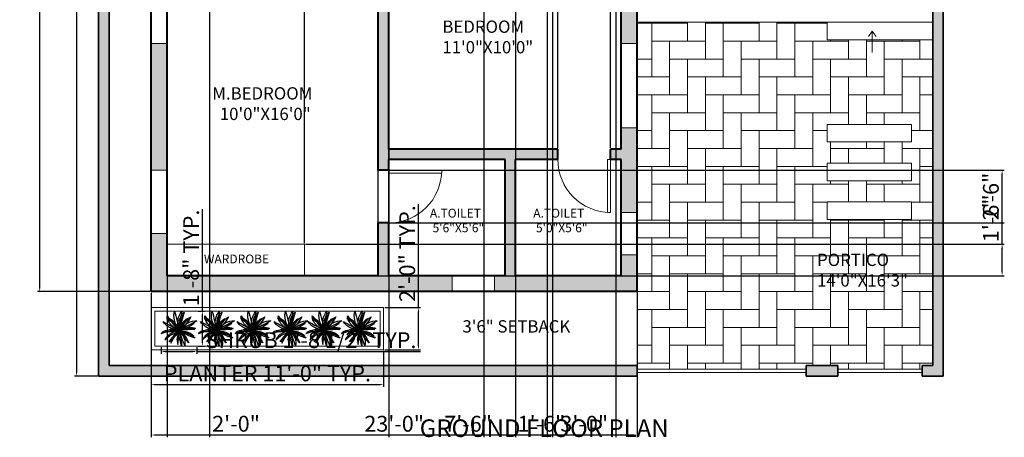
# Model space of a CAD drawing. Units: inches. Extents: x 2337 to 3570, y 1258 to 1938.
# Tile 20 of 30: x 2943 to 3502, y 1258 to 1496. Entities that reach past the tile are written whole.
import ezdxf

# ---------------------------------------------------------------- set-up
doc = ezdxf.new("R2010")
doc.units = ezdxf.units.IN
for name, color, linetype, lineweight in [('A-ANNO-DIMS', 2, 'Continuous', 18), ('A-ANNO-SYMB', 7, 'Continuous', 18), ('A-ANNO-TEXT', 7, 'Continuous', 18), ('A-ANNO-TITL', 7, 'Continuous', 30), ('A-AREA-IDEN', 7, 'Continuous', 18), ('A-DOOR', 4, 'Continuous', 20), ('A-FLOR-CASE', 34, 'Continuous', 18), ('A-FLOR-EDGE', 8, 'Continuous', 20), ('A-FLOR-PATT', 252, 'Continuous', 13), ('A-FLOR-STRS', 7, 'Continuous', 20), ('A-GLAZ', 4, 'Continuous', 18), ('A-WALL', 7, 'Continuous', 40), ('C-PROP', 7, 'Continuous', 35), ('CAY', 94, 'Continuous', 13), ('L-PLNT-BEDS', 94, 'Continuous', 20), ('L-SITE-GATE', 4, 'Continuous', 18)]:
    doc.layers.add(name, color=color, linetype=linetype, lineweight=lineweight)
doc.layers.add('A-WALL-PATT', color=18, linetype='Continuous', lineweight=13, true_color=0x000000)
doc.layers.add('C-PROP-PATT', color=251, linetype='Continuous', lineweight=13, true_color=0x636466)
doc.layers.add('DIENHOA', color=3, linetype='Continuous')
doc.styles.get("Standard").update_dxf_attribs({"font": 'arial.ttf'})
doc.dimstyles.new('ISO-25', dxfattribs={"dimtxt": 9, "dimasz": 2.5, "dimexe": 1.25, "dimexo": 0.625, "dimtad": 1, "dimdec": 1, "dimlunit": 3, "dimtxsty": 'Standard', "dimcen": 2.5, "dimadec": 0, "dimazin": 0, "dimtfac": 1, "dimtdec": 1, "dimtmove": 0, "dimatfit": 3, "dimfxl": 1, "dimarcsym": 0})

# ---------------------------------------------------------------- blocks, each defined once
blk = doc.blocks.new('*U3')
for p, q in [((0, 0), (0, -6)), ((30, 0), (30, -6))]:
    blk.add_line(p, q)
blk.add_lwpolyline([(0, 0), (0, 30), (1.75, 30), (1.75, 0)], close=True)
blk.add_arc((0, 0), 30, 0, 90)
blk = doc.blocks.new('*D5')
at = {"layer": 'A-ANNO-DIMS', "color": 0, "lineweight": -2, "transparency": 16777216}
for p, q in [((2987.16, 1893.12), (2974.1, 1893.12)), ((2975.35, 1890.62), (2975.35, 1295.62)), ((2987.16, 1293.12), (2974.1, 1293.12))]:
    blk.add_line(p, q, dxfattribs=at)
at = {"layer": 'A-ANNO-DIMS', "color": 0, "transparency": 16777216}
for points in [[(2974.93, 1890.62), (2975.77, 1890.62), (2975.35, 1893.12)], [(2974.93, 1295.62), (2975.77, 1295.62), (2975.35, 1293.12)]]:
    blk.add_solid(points, dxfattribs=at)
at = {"layer": 'Defpoints', "color": 0, "transparency": 16777216}
for p in [(2987.79, 1893.12), (2975.35, 1293.12), (2987.79, 1293.12)]:
    blk.add_point(p, dxfattribs=at)
at = {"layer": 'A-ANNO-DIMS', "color": 0, "transparency": 16777216, "insert": (2970.13, 1593.12), "char_height": 9, "attachment_point": 5, "rotation": 90}
blk.add_mtext("50'", dxfattribs=at)
blk = doc.blocks.new('Cay03_mb')
at = {"layer": 'DIENHOA'}
for p, q in [((-365, 390), (-414, 403)), ((-414, 403), (-240, 278)), ((-315, 371), (-365, 390)), ((-264, 343), (-315, 371)), ((-211, 305), (-264, 343)), ((10, 295), (25, 374)), ((25, 374), (49, 444)), ((49, 444), (79, 504)), ((97, 366), (76, 291)), ((79, 504), (119, 555)), ((119, 442), (97, 366)), ((119, 555), (166, 599)), ((142, 519), (119, 442)), ((166, 599), (142, 519)), ((-345, 5), (-400, -17)), ((-299, 20), (-345, 5)), ((-255, 27), (-299, 20)), ((-208, 28), (-255, 27)), ((-240, 278), (-88, 95)), ((-158, 252), (-211, 305)), ((-153, 22), (-208, 28)), ((-104, 184), (-158, 252)), ((-83, 10), (-153, 22)), ((-50, 98), (-104, 184)), ((-88, 95), (5, -8)), ((5, -8), (-83, 10)), ((5, -8), (-50, 98)), ((0, 105), (2, 206)), ((5, -8), (0, 105)), ((2, 206), (10, 295)), ((5, -8), (76, 75)), ((20, 68), (5, -8)), ((75, 36), (5, -8)), ((5, -8), (100, 18)), ((46, 1), (5, -8)), ((37, 142), (20, 68)), ((56, 216), (37, 142)), ((97, 7), (46, 1)), ((76, 291), (56, 216)), ((145, 77), (75, 36)), ((76, 75), (147, 144)), ((155, 12), (97, 7)), ((100, 18), (182, 37)), ((217, 117), (145, 77)), ((147, 144), (219, 200)), ((220, 15), (155, 12)), ((182, 37), (253, 49)), ((290, 155), (217, 117)), ((219, 200), (291, 243)), ((289, 17), (220, 15)), ((253, 49), (315, 54)), ((362, 19), (289, 17)), ((364, 193), (290, 155)), ((291, 243), (363, 275)), ((315, 54), (369, 53)), ((436, 19), (362, 19)), ((363, 275), (437, 297)), ((438, 231), (364, 193)), ((369, 53), (419, 47)), ((419, 47), (465, 35)), ((510, 19), (436, 19)), ((437, 297), (511, 310)), ((512, 271), (438, 231)), ((465, 35), (510, 19)), ((511, 310), (586, 314)), ((586, 314), (512, 271)), ((-400, -17), (-468, -48)), ((-468, -48), (-376, -38)), ((-376, -38), (-295, -28)), ((-330, -387), (-271, -307)), ((-295, -28), (-226, -19)), ((-250, -318), (-291, -355)), ((-271, -307), (-216, -236)), ((-206, -276), (-250, -318)), ((-226, -19), (-166, -11)), ((-216, -236), (-166, -174)), ((-162, -231), (-206, -276)), ((-166, -11), (-114, -6)), ((-166, -174), (-120, -122)), ((-118, -181), (-162, -231)), ((-120, -122), (-80, -80)), ((-75, -127), (-118, -181)), ((-114, -6), (-69, -3)), ((-80, -80), (-45, -46)), ((-33, -69), (-75, -127)), ((-69, -3), (-30, -3)), ((-45, -46), (-17, -22)), ((5, -8), (-33, -69)), ((-30, -3), (5, -8)), ((-17, -22), (5, -8)), ((5, -8), (57, -73)), ((26, -64), (5, -8)), ((5, -8), (113, -40)), ((53, -42), (5, -8)), ((47, -126), (26, -64)), ((69, -191), (47, -126)), ((107, -76), (53, -42)), ((57, -73), (100, -139)), ((91, -257), (69, -191)), ((113, -322), (91, -257)), ((100, -139), (136, -204)), ((166, -110), (107, -76)), ((113, -40), (207, -74)), ((135, -386), (113, -322)), ((136, -204), (163, -268)), ((163, -268), (181, -330)), ((229, -143), (166, -110)), ((207, -74), (290, -108)), ((296, -175), (229, -143)), ((290, -108), (359, -141)), ((367, -205), (296, -175)), ((359, -141), (417, -174)), ((442, -233), (367, -205)), ((417, -174), (463, -204)), ((519, -258), (442, -233)), ((463, -204), (496, -232)), ((496, -232), (519, -258)), ((-291, -355), (-330, -387)), ((158, -445), (135, -386)), ((180, -499), (158, -445)), ((190, -446), (180, -499)), ((181, -330), (190, -390)), ((190, -390), (190, -446))]:
    blk.add_line(p, q, dxfattribs=at)
for points in [[(-396, 474), (-348, 406), (-301, 339), (-254, 275), (-208, 212), (-162, 151), (-115, 91), (-66, 32), (-16, -27)], [(-16, -27), (-108, 39), (-187, 102), (-252, 163), (-305, 224), (-345, 285), (-374, 347), (-390, 409), (-396, 474)], [(24, -5), (-41, 82), (-92, 167), (-130, 249), (-156, 330), (-170, 408), (-175, 484), (-170, 559), (-157, 633)], [(-157, 633), (-132, 551), (-111, 470), (-90, 389), (-70, 309), (-49, 229), (-27, 150), (-3, 72), (24, -5)], [(-16, -27), (-38, 80), (-49, 178), (-49, 269), (-39, 353), (-19, 430), (9, 501), (45, 567), (88, 629)], [(88, 629), (75, 544), (61, 461), (46, 379), (31, 298), (16, 217), (3, 136), (-8, 55), (-16, -27)], [(273, 387), (228, 329), (182, 270), (138, 212), (97, 156), (60, 103), (28, 55), (2, 11), (-16, -27)], [(-16, -27), (21, 64), (57, 140), (91, 203), (125, 255), (160, 297), (195, 332), (233, 362), (273, 387)], [(24, -5), (20, 93), (20, 177), (25, 249), (34, 310), (47, 363), (65, 409), (87, 452), (113, 492)], [(113, 492), (96, 420), (79, 347), (64, 276), (50, 208), (38, 145), (30, 87), (25, 36), (24, -5)], [(384, 437), (342, 368), (298, 302), (253, 239), (206, 181), (159, 127), (113, 78), (68, 34), (24, -5)], [(24, -5), (80, 92), (134, 176), (186, 248), (234, 309), (279, 357), (319, 395), (355, 421), (384, 437)], [(-16, -27), (-134, -5), (-235, 5), (-322, 5), (-396, -5), (-459, -22), (-512, -46), (-558, -74), (-598, -105)], [(-530, 290), (-458, 248), (-388, 208), (-319, 169), (-251, 131), (-183, 95), (-115, 60), (-46, 26), (24, -5)], [(24, -5), (-87, 15), (-185, 40), (-270, 68), (-344, 101), (-406, 140), (-457, 184), (-499, 233), (-530, 290)], [(497, 224), (429, 178), (362, 137), (294, 99), (227, 66), (162, 37), (100, 11), (40, -10), (-16, -27)], [(-16, -27), (75, 38), (160, 92), (237, 136), (307, 170), (368, 195), (420, 213), (463, 222), (497, 224)], [(24, -5), (99, 30), (173, 57), (245, 77), (313, 88), (378, 92), (438, 87), (493, 74), (541, 52)], [(541, 52), (484, 43), (421, 35), (354, 28), (285, 21), (216, 14), (148, 8), (83, 2), (24, -5)], [(-598, -105), (-393, -44), (-155, -37), (-16, -27)], [(-472, -320), (-310, -179), (-98, -73), (24, -5)], [(24, -5), (-92, -35), (-188, -68), (-267, -105), (-330, -145), (-380, -187), (-418, -231), (-448, -275), (-472, -320)], [(-276, -424), (-227, -345), (-186, -276), (-150, -216), (-119, -164), (-91, -120), (-66, -82), (-41, -52), (-16, -27)], [(-16, -27), (-85, -86), (-137, -133), (-176, -173), (-204, -210), (-226, -249), (-243, -295), (-258, -352), (-276, -424)], [(24, -5), (-14, -88), (-41, -153), (-60, -205), (-70, -251), (-73, -295), (-69, -344), (-60, -402), (-45, -475)], [(-45, -475), (-34, -383), (-25, -303), (-18, -233), (-12, -173), (-6, -121), (2, -77), (11, -39), (24, -5)], [(76, -524), (49, -428), (27, -342), (9, -264), (-4, -196), (-12, -138), (-17, -90), (-18, -53), (-16, -27)], [(478, -192), (422, -176), (361, -157), (298, -135), (232, -113), (167, -89), (102, -67), (41, -45), (-16, -27)], [(-16, -27), (67, -27), (146, -33), (219, -45), (286, -63), (346, -87), (398, -117), (443, -152), (478, -192)], [(-16, -27), (8, -95), (29, -163), (44, -231), (56, -296), (65, -359), (71, -419), (74, -474), (76, -524)], [(316, -418), (251, -343), (195, -273), (147, -210), (106, -154), (74, -105), (50, -63), (33, -30), (24, -5)], [(24, -5), (75, -57), (122, -111), (164, -165), (203, -219), (237, -273), (267, -324), (294, -373), (316, -418)]]:
    blk.add_lwpolyline(points, dxfattribs=at)
blk = doc.blocks.new('STAIR-UP-ARROW')
for p, q in [((2.25, 12), (2.25, 0)), ((2.25, 0), (0, 3.01)), ((2.25, 0), (4.5, 3.01))]:
    blk.add_line(p, q)
blk = doc.blocks.new('PLANTER-132X24IN')
for points in [[(0, 24), (132, 24), (132, 0), (0, 0)], [(2, 22), (130, 22), (130, 2), (2, 2)]]:
    blk.add_lwpolyline(points, close=True)
blk = doc.blocks.new('*D46')
at = {"layer": 'A-ANNO-DIMS', "color": 0, "lineweight": -2, "transparency": 16777216}
for p, q in [((3023.35, 1309.55), (3023.35, 1305.87)), ((3043.75, 1309.55), (3043.75, 1305.87)), ((3025.85, 1307.12), (3041.25, 1307.12)), ((3043.75, 1307.12), (3170.8, 1307.12))]:
    blk.add_line(p, q, dxfattribs=at)
at = {"layer": 'A-ANNO-DIMS', "color": 0, "transparency": 16777216}
for points in [[(3025.85, 1307.54), (3025.85, 1306.7), (3023.35, 1307.12)], [(3041.25, 1307.54), (3041.25, 1306.7), (3043.75, 1307.12)]]:
    blk.add_solid(points, dxfattribs=at)
at = {"layer": 'Defpoints', "color": 0, "transparency": 16777216}
for p in [(3023.35, 1310.18), (3043.75, 1310.18), (3043.75, 1307.12)]:
    blk.add_point(p, dxfattribs=at)
at = {"layer": 'A-ANNO-DIMS', "color": 0, "transparency": 16777216, "insert": (3108.53, 1312.4), "char_height": 9, "attachment_point": 5}
blk.add_mtext('SHRUB 1\'-8 1/2" TYP.', dxfattribs=at)
blk = doc.blocks.new('*D47')
at = {"layer": 'A-ANNO-DIMS', "color": 0, "lineweight": -2, "transparency": 16777216}
for p, q in [((3046.81, 1330.12), (3046.81, 1387.88)), ((3044.38, 1330.12), (3048.06, 1330.12)), ((3046.81, 1312.68), (3046.81, 1327.62)), ((3044.38, 1310.18), (3048.06, 1310.18))]:
    blk.add_line(p, q, dxfattribs=at)
at = {"layer": 'A-ANNO-DIMS', "color": 0, "transparency": 16777216}
for points in [[(3046.4, 1327.62), (3047.23, 1327.62), (3046.81, 1330.12)], [(3046.4, 1312.68), (3047.23, 1312.68), (3046.81, 1310.18)]]:
    blk.add_solid(points, dxfattribs=at)
at = {"layer": 'Defpoints', "color": 0, "transparency": 16777216}
for p in [(3043.75, 1330.12), (3046.81, 1330.12), (3043.75, 1310.18)]:
    blk.add_point(p, dxfattribs=at)
at = {"layer": 'A-ANNO-DIMS', "color": 0, "transparency": 16777216, "insert": (3041.59, 1360.25), "char_height": 9, "attachment_point": 5, "rotation": 90}
blk.add_mtext('1\'-8" TYP.', dxfattribs=at)
blk = doc.blocks.new('*D74')
at = {"layer": 'A-ANNO-DIMS', "color": 0, "lineweight": -2, "transparency": 16777216}
for p, q in [((3017.79, 1307.49), (3017.79, 1287.07)), ((3149.79, 1307.49), (3149.79, 1287.07)), ((3020.29, 1288.32), (3147.29, 1288.32))]:
    blk.add_line(p, q, dxfattribs=at)
at = {"layer": 'A-ANNO-DIMS', "color": 0, "transparency": 16777216}
for points in [[(3020.29, 1288.73), (3020.29, 1287.9), (3017.79, 1288.32)], [(3147.29, 1288.73), (3147.29, 1287.9), (3149.79, 1288.32)]]:
    blk.add_solid(points, dxfattribs=at)
at = {"layer": 'Defpoints', "color": 0, "transparency": 16777216}
for p in [(3017.79, 1308.12), (3149.79, 1308.12), (3149.79, 1288.32)]:
    blk.add_point(p, dxfattribs=at)
at = {"layer": 'A-ANNO-DIMS', "color": 0, "transparency": 16777216, "insert": (3083.79, 1293.54), "char_height": 9, "attachment_point": 5}
blk.add_mtext('PLANTER 11\'-0" TYP.', dxfattribs=at)
blk = doc.blocks.new('*D75')
at = {"layer": 'A-ANNO-DIMS', "color": 0, "lineweight": -2, "transparency": 16777216}
for p, q in [((3169.59, 1332.12), (3169.59, 1390.88)), ((3150.41, 1332.12), (3170.84, 1332.12)), ((3169.59, 1310.62), (3169.59, 1329.62)), ((3150.41, 1308.12), (3170.84, 1308.12))]:
    blk.add_line(p, q, dxfattribs=at)
at = {"layer": 'A-ANNO-DIMS', "color": 0, "transparency": 16777216}
for points in [[(3169.17, 1329.62), (3170, 1329.62), (3169.59, 1332.12)], [(3169.17, 1310.62), (3170, 1310.62), (3169.59, 1308.12)]]:
    blk.add_solid(points, dxfattribs=at)
at = {"layer": 'Defpoints', "color": 0, "transparency": 16777216}
for p in [(3149.79, 1332.12), (3169.59, 1332.12), (3149.79, 1308.12)]:
    blk.add_point(p, dxfattribs=at)
at = {"layer": 'A-ANNO-DIMS', "color": 0, "transparency": 16777216, "insert": (3164.37, 1362.75), "char_height": 9, "attachment_point": 5, "rotation": 90}
blk.add_mtext('2\'-0" TYP.', dxfattribs=at)
blk = doc.blocks.new('*D100')
at = {"layer": 'A-ANNO-DIMS', "color": 0, "lineweight": -2, "transparency": 16777216}
for p, q in [((3248.79, 1422.74), (3248.79, 1927.77)), ((3251.29, 1926.52), (3276.29, 1926.52)), ((3278.79, 1422.74), (3278.79, 1927.77))]:
    blk.add_line(p, q, dxfattribs=at)
at = {"layer": 'A-ANNO-DIMS', "color": 0, "transparency": 16777216}
for points in [[(3251.29, 1926.93), (3251.29, 1926.1), (3248.79, 1926.52)], [(3276.29, 1926.93), (3276.29, 1926.1), (3278.79, 1926.52)]]:
    blk.add_solid(points, dxfattribs=at)
at = {"layer": 'Defpoints', "color": 0, "transparency": 16777216}
for p in [(3278.79, 1926.52), (3248.79, 1422.12), (3278.79, 1422.12)]:
    blk.add_point(p, dxfattribs=at)
at = {"layer": 'A-ANNO-DIMS', "color": 0, "transparency": 16777216, "insert": (3263.79, 1931.74), "char_height": 9, "attachment_point": 5}
blk.add_mtext('2\'-6"', dxfattribs=at)
blk = doc.blocks.new('*D101')
at = {"layer": 'A-ANNO-DIMS', "color": 0, "lineweight": -2, "transparency": 16777216}
for p, q in [((3147.41, 1410.12), (3502.44, 1410.12)), ((3501.19, 1382.62), (3501.19, 1407.62)), ((3147.41, 1380.12), (3502.44, 1380.12))]:
    blk.add_line(p, q, dxfattribs=at)
at = {"layer": 'A-ANNO-DIMS', "color": 0, "transparency": 16777216}
for points in [[(3500.77, 1407.62), (3501.6, 1407.62), (3501.19, 1410.12)], [(3500.77, 1382.62), (3501.6, 1382.62), (3501.19, 1380.12)]]:
    blk.add_solid(points, dxfattribs=at)
at = {"layer": 'Defpoints', "color": 0, "transparency": 16777216}
for p in [(3146.79, 1410.12), (3501.19, 1410.12), (3146.79, 1380.12)]:
    blk.add_point(p, dxfattribs=at)
at = {"layer": 'A-ANNO-DIMS', "color": 0, "transparency": 16777216, "insert": (3495.97, 1395.12), "char_height": 9, "attachment_point": 5, "rotation": 90}
blk.add_mtext('2\'-6"', dxfattribs=at)
blk = doc.blocks.new('*D102')
at = {"layer": 'A-ANNO-DIMS', "color": 0, "lineweight": -2, "transparency": 16777216}
for p, q in [((3245.79, 1763.49), (3245.79, 1258.47)), ((3281.79, 1763.49), (3281.79, 1258.47)), ((3248.29, 1259.72), (3279.29, 1259.72))]:
    blk.add_line(p, q, dxfattribs=at)
at = {"layer": 'A-ANNO-DIMS', "color": 0, "transparency": 16777216}
for points in [[(3248.29, 1260.13), (3248.29, 1259.3), (3245.79, 1259.72)], [(3279.29, 1260.13), (3279.29, 1259.3), (3281.79, 1259.72)]]:
    blk.add_solid(points, dxfattribs=at)
at = {"layer": 'Defpoints', "color": 0, "transparency": 16777216}
for p in [(3245.79, 1764.12), (3281.79, 1764.12), (3281.79, 1259.72)]:
    blk.add_point(p, dxfattribs=at)
at = {"layer": 'A-ANNO-DIMS', "color": 0, "transparency": 16777216, "insert": (3263.79, 1264.94), "char_height": 9, "attachment_point": 5}
blk.add_mtext('3\'-0"', dxfattribs=at)
blk = doc.blocks.new('*D104')
at = {"layer": 'A-ANNO-DIMS', "color": 0, "lineweight": -2, "transparency": 16777216}
for p, q in [((3144.29, 1926.52), (3141.79, 1926.52)), ((3146.79, 1350.74), (3146.79, 1927.77)), ((3146.79, 1926.52), (3152.79, 1926.52)), ((3152.79, 1350.74), (3152.79, 1927.77)), ((3155.29, 1926.52), (3182.96, 1926.52))]:
    blk.add_line(p, q, dxfattribs=at)
at = {"layer": 'A-ANNO-DIMS', "color": 0, "transparency": 16777216}
for points in [[(3144.29, 1926.93), (3144.29, 1926.1), (3146.79, 1926.52)], [(3155.29, 1926.93), (3155.29, 1926.1), (3152.79, 1926.52)]]:
    blk.add_solid(points, dxfattribs=at)
at = {"layer": 'Defpoints', "color": 0, "transparency": 16777216}
for p in [(3152.79, 1926.52), (3146.79, 1350.12), (3152.79, 1350.12)]:
    blk.add_point(p, dxfattribs=at)
at = {"layer": 'A-ANNO-DIMS', "color": 0, "transparency": 16777216, "insert": (3170.37, 1931.74), "char_height": 9, "attachment_point": 5}
blk.add_mtext('0\'-6"', dxfattribs=at)
blk = doc.blocks.new('*D105')
at = {"layer": 'A-ANNO-DIMS', "color": 0, "lineweight": -2, "transparency": 16777216}
for p, q in [((3026.79, 1640.49), (3026.79, 1258.47)), ((3050.79, 1640.49), (3050.79, 1258.47)), ((3029.29, 1259.72), (3048.29, 1259.72)), ((3050.79, 1259.72), (3078.61, 1259.72))]:
    blk.add_line(p, q, dxfattribs=at)
at = {"layer": 'A-ANNO-DIMS', "color": 0, "transparency": 16777216}
for points in [[(3029.29, 1260.13), (3029.29, 1259.3), (3026.79, 1259.72)], [(3048.29, 1260.13), (3048.29, 1259.3), (3050.79, 1259.72)]]:
    blk.add_solid(points, dxfattribs=at)
at = {"layer": 'Defpoints', "color": 0, "transparency": 16777216}
for p in [(3026.79, 1641.12), (3050.79, 1641.12), (3050.79, 1259.72)]:
    blk.add_point(p, dxfattribs=at)
at = {"layer": 'A-ANNO-DIMS', "color": 0, "transparency": 16777216, "insert": (3065.95, 1264.94), "char_height": 9, "attachment_point": 5}
blk.add_mtext('2\'-0"', dxfattribs=at)
blk = doc.blocks.new('*D109')
at = {"layer": 'A-ANNO-DIMS', "color": 0, "lineweight": -2, "transparency": 16777216}
for p, q in [((3017.79, 1340.49), (3017.79, 1258.47)), ((3293.79, 1340.49), (3293.79, 1258.47)), ((3020.29, 1259.72), (3291.29, 1259.72))]:
    blk.add_line(p, q, dxfattribs=at)
at = {"layer": 'A-ANNO-DIMS', "color": 0, "transparency": 16777216}
for points in [[(3020.29, 1260.13), (3020.29, 1259.3), (3017.79, 1259.72)], [(3291.29, 1260.13), (3291.29, 1259.3), (3293.79, 1259.72)]]:
    blk.add_solid(points, dxfattribs=at)
at = {"layer": 'Defpoints', "color": 0, "transparency": 16777216}
for p in [(3017.79, 1341.12), (3293.79, 1341.12), (3293.79, 1259.72)]:
    blk.add_point(p, dxfattribs=at)
at = {"layer": 'A-ANNO-DIMS', "color": 0, "transparency": 16777216, "insert": (3155.79, 1264.94), "char_height": 9, "attachment_point": 5}
blk.add_mtext('23\'-0"', dxfattribs=at)
blk = doc.blocks.new('*D110')
at = {"layer": 'A-ANNO-DIMS', "color": 0, "lineweight": -2, "transparency": 16777216}
for p, q in [((3017.16, 1857.12), (2953.14, 1857.12)), ((2954.39, 1343.62), (2954.39, 1854.62)), ((3017.16, 1341.12), (2953.14, 1341.12))]:
    blk.add_line(p, q, dxfattribs=at)
at = {"layer": 'A-ANNO-DIMS', "color": 0, "transparency": 16777216}
for points in [[(2953.97, 1854.62), (2954.8, 1854.62), (2954.39, 1857.12)], [(2953.97, 1343.62), (2954.8, 1343.62), (2954.39, 1341.12)]]:
    blk.add_solid(points, dxfattribs=at)
at = {"layer": 'Defpoints', "color": 0, "transparency": 16777216}
for p in [(2954.39, 1857.12), (3017.79, 1857.12), (3017.79, 1341.12)]:
    blk.add_point(p, dxfattribs=at)
at = {"layer": 'A-ANNO-DIMS', "color": 0, "transparency": 16777216, "insert": (2949.16, 1599.12), "char_height": 9, "attachment_point": 5, "rotation": 90}
blk.add_mtext('43\'-0"', dxfattribs=at)
blk = doc.blocks.new('*D112')
at = {"layer": 'A-ANNO-DIMS', "color": 0, "lineweight": -2, "transparency": 16777216}
for p, q in [((3026.79, 1368.74), (3026.79, 1927.77)), ((3029.29, 1926.52), (3102.29, 1926.52)), ((3104.79, 1368.74), (3104.79, 1927.77))]:
    blk.add_line(p, q, dxfattribs=at)
at = {"layer": 'A-ANNO-DIMS', "color": 0, "transparency": 16777216}
for points in [[(3029.29, 1926.93), (3029.29, 1926.1), (3026.79, 1926.52)], [(3102.29, 1926.93), (3102.29, 1926.1), (3104.79, 1926.52)]]:
    blk.add_solid(points, dxfattribs=at)
at = {"layer": 'Defpoints', "color": 0, "transparency": 16777216}
for p in [(3104.79, 1926.52), (3026.79, 1368.12), (3104.79, 1368.12)]:
    blk.add_point(p, dxfattribs=at)
at = {"layer": 'A-ANNO-DIMS', "color": 0, "transparency": 16777216, "insert": (3065.79, 1931.74), "char_height": 9, "attachment_point": 5}
blk.add_mtext('6\'-6"', dxfattribs=at)
blk = doc.blocks.new('*D113')
at = {"layer": 'A-ANNO-DIMS', "color": 0, "lineweight": -2, "transparency": 16777216}
for p, q in [((3501.19, 1368.12), (3501.19, 1394.94)), ((3105.41, 1368.12), (3502.44, 1368.12)), ((3501.19, 1352.62), (3501.19, 1365.62)), ((3105.41, 1350.12), (3502.44, 1350.12))]:
    blk.add_line(p, q, dxfattribs=at)
at = {"layer": 'A-ANNO-DIMS', "color": 0, "transparency": 16777216}
for points in [[(3500.77, 1365.62), (3501.6, 1365.62), (3501.19, 1368.12)], [(3500.77, 1352.62), (3501.6, 1352.62), (3501.19, 1350.12)]]:
    blk.add_solid(points, dxfattribs=at)
at = {"layer": 'Defpoints', "color": 0, "transparency": 16777216}
for p in [(3104.79, 1368.12), (3501.19, 1368.12), (3104.79, 1350.12)]:
    blk.add_point(p, dxfattribs=at)
at = {"layer": 'A-ANNO-DIMS', "color": 0, "transparency": 16777216, "insert": (3495.97, 1382.78), "char_height": 9, "attachment_point": 5, "rotation": 90}
blk.add_mtext('1\'-6"', dxfattribs=at)
blk = doc.blocks.new('*D114')
at = {"layer": 'A-ANNO-DIMS', "color": 0, "lineweight": -2, "transparency": 16777216}
for p, q in [((3152.79, 1523.49), (3152.79, 1258.47)), ((3242.79, 1523.49), (3242.79, 1258.47)), ((3155.29, 1259.72), (3240.29, 1259.72))]:
    blk.add_line(p, q, dxfattribs=at)
at = {"layer": 'A-ANNO-DIMS', "color": 0, "transparency": 16777216}
for points in [[(3155.29, 1260.13), (3155.29, 1259.3), (3152.79, 1259.72)], [(3240.29, 1260.13), (3240.29, 1259.3), (3242.79, 1259.72)]]:
    blk.add_solid(points, dxfattribs=at)
at = {"layer": 'Defpoints', "color": 0, "transparency": 16777216}
for p in [(3152.79, 1524.12), (3242.79, 1524.12), (3242.79, 1259.72)]:
    blk.add_point(p, dxfattribs=at)
at = {"layer": 'A-ANNO-DIMS', "color": 0, "transparency": 16777216, "insert": (3197.79, 1264.94), "char_height": 9, "attachment_point": 5}
blk.add_mtext('7\'-6"', dxfattribs=at)
blk = doc.blocks.new('*D117')
at = {"layer": 'A-ANNO-DIMS', "color": 0, "lineweight": -2, "transparency": 16777216}
for p, q in [((3206.79, 1604.49), (3206.79, 1258.47)), ((3224.79, 1604.49), (3224.79, 1258.47)), ((3209.29, 1259.72), (3222.29, 1259.72)), ((3224.79, 1259.72), (3251.61, 1259.72))]:
    blk.add_line(p, q, dxfattribs=at)
at = {"layer": 'A-ANNO-DIMS', "color": 0, "transparency": 16777216}
for points in [[(3209.29, 1260.13), (3209.29, 1259.3), (3206.79, 1259.72)], [(3222.29, 1260.13), (3222.29, 1259.3), (3224.79, 1259.72)]]:
    blk.add_solid(points, dxfattribs=at)
at = {"layer": 'Defpoints', "color": 0, "transparency": 16777216}
for p in [(3206.79, 1605.12), (3224.79, 1605.12), (3224.79, 1259.72)]:
    blk.add_point(p, dxfattribs=at)
at = {"layer": 'A-ANNO-DIMS', "color": 0, "transparency": 16777216, "insert": (3239.45, 1264.94), "char_height": 9, "attachment_point": 5}
blk.add_mtext('1\'-6"', dxfattribs=at)

msp = doc.modelspace()

# ---------------------------------------------------------------- hatches: boundary and pattern name
at = {"layer": 'A-FLOR-PATT'}
h = msp.add_hatch(dxfattribs=at)
h.set_pattern_fill('AR-HBONE', color=256, scale=0.1, angle=45)
h.set_pattern_definition([(90, (-558.681, 0), (-10.16, 10.16), [30.48, -10.16]), (180, (-558.681, 10.16), (-10.16, 10.16), [30.48, -10.16])])
h.paths.add_polyline_path([(3461.79, 1484.12), (3401.79, 1484.12), (3401.79, 1494.12), (3293.79, 1494.12), (3293.79, 1341.12), (3293.79, 1299.12), (3293.79, 1297.12), (3389.79, 1297.12), (3389.79, 1299.12), (3407.79, 1299.12), (3407.79, 1297.12), (3455.79, 1297.12), (3455.79, 1299.12), (3461.79, 1299.12)])
h.paths.add_polyline_path([(3401.79, 1426.12), (3401.79, 1436.12), (3449.79, 1436.12), (3449.79, 1426.12)], flags=16)
h.paths.add_polyline_path([(3401.79, 1414.12), (3449.79, 1414.12), (3449.79, 1404.12), (3401.79, 1404.12)], flags=16)
h.paths.add_polyline_path([(3401.79, 1392.12), (3449.79, 1392.12), (3449.79, 1382.12), (3401.79, 1382.12)], flags=16)
h.paths.add_polyline_path([(3393.24, 1340.04), (3446.57, 1340.04), (3446.57, 1366.16), (3393.24, 1366.16)], flags=24)
at = {"layer": 'A-WALL-PATT'}
h = msp.add_hatch(color=256, dxfattribs=at)
h.dxf.hatch_style = 1
h.paths.add_polyline_path([(3233.79, 1857.12), (3017.79, 1857.12), (3017.79, 1824.12), (3026.79, 1824.12), (3026.79, 1848.12), (3233.79, 1848.12)])
h.paths.add_polyline_path([(3128.79, 1764.12), (3026.79, 1764.12), (3026.79, 1788.12), (3017.79, 1788.12), (3017.79, 1743.12), (3026.79, 1743.12), (3026.79, 1755.12), (3128.79, 1755.12)])
h.paths.add_polyline_path([(3245.79, 1761.12), (3245.79, 1764.12), (3164.79, 1764.12), (3164.79, 1755.12), (3170.79, 1755.12), (3170.79, 1701.12), (3224.79, 1701.12), (3224.79, 1605.12), (3233.79, 1605.12), (3233.79, 1713.12), (3224.79, 1713.12), (3224.79, 1707.12), (3176.79, 1707.12), (3176.79, 1755.12), (3224.79, 1755.12), (3224.79, 1749.12), (3233.79, 1749.12), (3233.79, 1755.12), (3245.79, 1755.12)])
h.paths.add_polyline_path([(3026.79, 1707.12), (3017.79, 1707.12), (3017.79, 1617.12), (3026.79, 1617.12), (3026.79, 1635.12), (3068.79, 1635.12), (3068.79, 1641.12), (3026.79, 1641.12)])
h.paths.add_polyline_path([(3104.79, 1551.12), (3026.79, 1551.12), (3026.79, 1569.12), (3017.79, 1569.12), (3017.79, 1518.12), (3026.79, 1518.12), (3026.79, 1542.12), (3104.79, 1542.12)])
h.paths.add_polyline_path([(3026.79, 1482.12), (3017.79, 1482.12), (3017.79, 1410.12), (3026.79, 1410.12)])
h.paths.add_polyline_path([(3188.79, 1350.12), (3152.79, 1350.12), (3152.79, 1380.12), (3146.79, 1380.12), (3146.79, 1350.12), (3026.79, 1350.12), (3026.79, 1374.12), (3017.79, 1374.12), (3017.79, 1341.12), (3188.79, 1341.12)])
h.paths.add_polyline_path([(3224.79, 1416.12), (3248.79, 1416.12), (3248.79, 1422.12), (3152.79, 1422.12), (3152.79, 1542.12), (3242.79, 1542.12), (3242.79, 1551.12), (3233.79, 1551.12), (3233.79, 1557.12), (3224.79, 1557.12), (3224.79, 1551.12), (3140.79, 1551.12), (3140.79, 1542.12), (3146.79, 1542.12), (3146.79, 1410.12), (3152.79, 1410.12), (3152.79, 1416.12), (3218.79, 1416.12), (3218.79, 1350.12), (3212.79, 1350.12), (3212.79, 1341.12), (3293.79, 1341.12), (3293.79, 1362.12), (3284.79, 1362.12), (3284.79, 1350.12), (3224.79, 1350.12)])
h.paths.add_polyline_path([(3293.79, 1434.12), (3284.79, 1434.12), (3284.79, 1422.12), (3278.79, 1422.12), (3278.79, 1416.12), (3284.79, 1416.12), (3284.79, 1386.12), (3293.79, 1386.12)], flags=17)
h.paths.add_polyline_path([(3293.79, 1542.12), (3314.79, 1542.12), (3314.79, 1551.12), (3278.79, 1551.12), (3278.79, 1545.12), (3278.79, 1542.12), (3284.79, 1542.12), (3284.79, 1482.12), (3293.79, 1482.12)])
h.paths.add_polyline_path([(3371.79, 1551.12), (3350.79, 1551.12), (3350.79, 1542.12), (3371.79, 1542.12), (3371.79, 1548.12)])
h.paths.add_polyline_path([(3434.79, 1647.12), (3425.79, 1647.12), (3425.79, 1551.12), (3419.79, 1551.12), (3419.79, 1548.12), (3419.79, 1542.12), (3434.79, 1542.12)])
h.paths.add_polyline_path([(3434.79, 1764.12), (3389.79, 1764.12), (3389.79, 1755.12), (3425.79, 1755.12), (3425.79, 1719.12), (3434.79, 1719.12)])
h.paths.add_polyline_path([(3317.79, 1764.12), (3281.79, 1764.12), (3281.79, 1755.12), (3317.79, 1755.12)])
at = {"layer": 'C-PROP-PATT'}
h = msp.add_hatch(color=256, dxfattribs=at)
h.dxf.hatch_style = 1
h.paths.add_polyline_path([(3467.79, 1893.12), (2987.79, 1893.12), (2987.79, 1293.12), (3293.79, 1293.12), (3293.79, 1299.12), (2993.79, 1299.12), (2993.79, 1887.12), (3461.79, 1887.12), (3461.79, 1875.12), (3467.79, 1875.12)])
h.paths.add_polyline_path([(3407.79, 1299.12), (3389.79, 1299.12), (3389.79, 1293.12), (3407.79, 1293.12)], flags=17)
h.paths.add_polyline_path([(3461.79, 1299.12), (3455.79, 1299.12), (3455.79, 1293.12), (3467.79, 1293.12), (3467.79, 1779.12), (3461.79, 1779.12)], flags=17)

# ---------------------------------------------------------------- linework, layer by layer
at = {"layer": 'A-FLOR-CASE'}
for q in [(3026.79, 1368.12), (3104.79, 1350.12)]:
    msp.add_line((3104.79, 1368.12), q, dxfattribs=at)
at = {"layer": 'A-FLOR-EDGE'}
for p, q in [((3461.79, 1494.12), (3293.79, 1494.12)), ((3293.79, 1341.12), (3293.79, 1299.12))]:
    msp.add_line(p, q, dxfattribs=at)
for points in [[(3401.79, 1436.12), (3449.79, 1436.12), (3449.79, 1426.12), (3401.79, 1426.12)], [(3401.79, 1414.12), (3449.79, 1414.12), (3449.79, 1404.12), (3401.79, 1404.12)], [(3401.79, 1392.12), (3449.79, 1392.12), (3449.79, 1382.12), (3401.79, 1382.12)]]:
    msp.add_lwpolyline(points, close=True, dxfattribs=at)
at = {"layer": 'A-FLOR-STRS'}
for p, q in [((3401.79, 1484.12), (3401.79, 1494.12)), ((3461.79, 1484.12), (3401.79, 1484.12))]:
    msp.add_line(p, q, dxfattribs=at)
at = {"layer": 'A-GLAZ'}
for p, q in [((3026.79, 1482.12), (3017.79, 1482.12)), ((3293.79, 1482.12), (3284.79, 1482.12)), ((3293.79, 1434.12), (3284.79, 1434.12)), ((3026.79, 1410.12), (3017.79, 1410.12)), ((3293.79, 1386.12), (3284.79, 1386.12)), ((3026.79, 1374.12), (3017.79, 1374.12)), ((3293.79, 1362.12), (3284.79, 1362.12)), ((3188.79, 1341.12), (3188.79, 1350.12)), ((3212.79, 1341.12), (3212.79, 1350.12))]:
    msp.add_line(p, q, dxfattribs=at)
at = {"layer": 'A-WALL'}
for p, q in [((3017.79, 1341.12), (3017.79, 1857.12)), ((3026.79, 1350.12), (3026.79, 1542.12)), ((3146.79, 1410.12), (3146.79, 1542.12)), ((3152.79, 1422.12), (3152.79, 1542.12)), ((3284.79, 1422.12), (3284.79, 1542.12)), ((3293.79, 1341.12), (3293.79, 1542.12)), ((3248.79, 1422.12), (3152.79, 1422.12)), ((3248.79, 1416.12), (3248.79, 1422.12)), ((3284.79, 1422.12), (3278.79, 1422.12)), ((3278.79, 1416.12), (3278.79, 1422.12)), ((3218.79, 1416.12), (3152.79, 1416.12)), ((3152.79, 1410.12), (3152.79, 1416.12)), ((3218.79, 1350.12), (3218.79, 1416.12)), ((3224.79, 1350.12), (3224.79, 1416.12)), ((3248.79, 1416.12), (3224.79, 1416.12)), ((3284.79, 1416.12), (3278.79, 1416.12)), ((3284.79, 1350.12), (3284.79, 1416.12)), ((3152.79, 1410.12), (3146.79, 1410.12)), ((3146.79, 1350.12), (3146.79, 1380.12)), ((3152.79, 1380.12), (3146.79, 1380.12)), ((3152.79, 1350.12), (3152.79, 1380.12)), ((3146.79, 1350.12), (3026.79, 1350.12)), ((3218.79, 1350.12), (3152.79, 1350.12)), ((3284.79, 1350.12), (3224.79, 1350.12)), ((3293.79, 1341.12), (3017.79, 1341.12))]:
    msp.add_line(p, q, dxfattribs=at)
at = {"layer": 'C-PROP'}
for p, q in [((2987.79, 1293.12), (2987.79, 1893.12)), ((2993.79, 1299.12), (2993.79, 1887.12)), ((3461.79, 1779.12), (3461.79, 1299.12)), ((3467.79, 1779.12), (3467.79, 1293.12)), ((3293.79, 1299.12), (2993.79, 1299.12)), ((3293.79, 1299.12), (3293.79, 1293.12)), ((3389.79, 1299.12), (3389.79, 1293.12)), ((3407.79, 1299.12), (3407.79, 1293.12)), ((3455.79, 1299.12), (3455.79, 1293.12)), ((3461.79, 1299.12), (3455.79, 1299.12)), ((3293.79, 1293.12), (2987.79, 1293.12)), ((3407.79, 1293.12), (3389.79, 1293.12)), ((3467.79, 1293.12), (3455.79, 1293.12))]:
    msp.add_line(p, q, dxfattribs=at)
msp.add_lwpolyline([(3407.79, 1299.12), (3389.79, 1299.12)], dxfattribs=at)
at = {"layer": 'L-SITE-GATE'}
for p, q in [((3293.79, 1297.12), (3389.79, 1297.12)), ((3293.79, 1295.12), (3389.79, 1295.12)), ((3407.79, 1297.12), (3455.79, 1297.12)), ((3407.79, 1295.12), (3455.79, 1295.12))]:
    msp.add_line(p, q, dxfattribs=at)

# ---------------------------------------------------------------- block references
at = {"layer": 'A-ANNO-SYMB', "rotation": 180}
msp.add_blockref('STAIR-UP-ARROW', (3429.7, 1488.98), dxfattribs=at)
at = {"layer": 'A-DOOR'}
for p, rotation in [((3278.79, 1416.12), 180), ((3152.79, 1410.12), 270)]:
    msp.add_blockref('*U3', p, dxfattribs=dict(at, rotation=rotation))
at = {"layer": 'CAY', "xscale": 0.0172255344823027, "yscale": 0.0172255344823027, "zscale": 0.0172255344823027}
for p in [(3033.66, 1319.21), (3054.97, 1319.21), (3075.66, 1319.21), (3096.7, 1319.21), (3116.05, 1319.21), (3136.11, 1319.21)]:
    msp.add_blockref('Cay03_mb', p, dxfattribs=at)
at = {"layer": 'L-PLNT-BEDS'}
msp.add_blockref('PLANTER-132X24IN', (3017.79, 1308.12), dxfattribs=at)

# ---------------------------------------------------------------- texts
at = {"layer": 'A-ANNO-TEXT', "attachment_point": 1}
for s, insert, char_height in [('WARDROBE', (3047.69, 1362.19), 5), ('3\'6" SETBACK', (3194.55, 1324.89), 7)]:
    msp.add_mtext_dynamic_manual_height_columns(s, width=66.911, gutter_width=12.5, heights=[0], dxfattribs=dict(at, insert=insert, char_height=char_height))
at = {"layer": 'A-ANNO-TITL', "insert": (3170.3, 1268.59), "char_height": 10, "attachment_point": 1}
msp.add_mtext_dynamic_manual_height_columns('GROUND FLOOR PLAN', width=180.1947, gutter_width=12.5, heights=[0], dxfattribs=at)
at = {"layer": 'A-AREA-IDEN', "attachment_point": 1}
for s, insert, char_height in [('BEDROOM     11\'0"X10\'0"', (3183.17, 1495.1), 7), ('M.BEDROOM\\P  10\'0"X16\'0"', (3052.45, 1457.23), 7), ('A.TOILET\\P 5\'6"X5\'6"', (3176.09, 1388.19), 5), ('A.TOILET\\P 5\'0"X5\'6"', (3234.82, 1388.19), 5), ('PORTICO\\P14\'0"X16\'3"', (3396.06, 1362.68), 7)]:
    msp.add_mtext_dynamic_manual_height_columns(s, width=66.911, gutter_width=12.5, heights=[0], dxfattribs=dict(at, insert=insert, char_height=char_height))

# ---------------------------------------------------------------- dimensions: what is measured, and where the dimension line sits
at = {"layer": 'A-ANNO-DIMS'}
for base, p1, p2, picture, middle in [((3104.79, 1926.52), (3026.79, 1368.12), (3104.79, 1368.12), '*D112', (3065.79, 1931.74)), ((3152.79, 1926.52), (3146.79, 1350.12), (3152.79, 1350.12), '*D104', (3170.37, 1931.74)), ((3278.79, 1926.52), (3248.79, 1422.12), (3278.79, 1422.12), '*D100', (3263.79, 1931.74)), ((3281.79, 1259.72), (3245.79, 1764.12), (3281.79, 1764.12), '*D102', (3263.79, 1264.94)), ((3050.79, 1259.72), (3026.79, 1641.12), (3050.79, 1641.12), '*D105', (3065.95, 1264.94)), ((3224.79, 1259.72), (3206.79, 1605.12), (3224.79, 1605.12), '*D117', (3239.45, 1264.94)), ((3242.79, 1259.72), (3152.79, 1524.12), (3242.79, 1524.12), '*D114', (3197.79, 1264.94)), ((3293.79, 1259.72), (3017.79, 1341.12), (3293.79, 1341.12), '*D109', (3155.79, 1264.94))]:
    dim = msp.add_linear_dim(base=base, p1=p1, p2=p2, dimstyle='ISO-25', override={"dimdec": 1, "dimlfac": 1, "dimrnd": 0, "dimzin": 1, "dimdsep": 46, "dimlunit": 4, "dimfrac": 2}, dxfattribs=at)
    dim.commit()
    dim.dimension.update_dxf_attribs({"geometry": picture, "text_midpoint": middle})
for base, p1, p2, override, picture, middle in [((2975.35, 1293.12), (2987.79, 1893.12), (2987.79, 1293.12), {"dimclrd": 0, "dimclre": 0, "dimclrt": 0}, '*D5', (2970.13, 1593.12)), ((2954.39, 1857.12), (3017.79, 1341.12), (3017.79, 1857.12), {"dimdec": 1, "dimlfac": 1, "dimrnd": 0, "dimzin": 1, "dimdsep": 46, "dimlunit": 4, "dimfrac": 2}, '*D110', (2949.16, 1599.12)), ((3501.19, 1410.12), (3146.79, 1380.12), (3146.79, 1410.12), {"dimdec": 1, "dimlfac": 1, "dimrnd": 0, "dimzin": 1, "dimdsep": 46, "dimlunit": 4, "dimfrac": 2}, '*D101', (3495.97, 1395.12)), ((3501.19, 1368.12), (3104.79, 1350.12), (3104.79, 1368.12), {"dimdec": 1, "dimlfac": 1, "dimrnd": 0, "dimzin": 1, "dimdsep": 46, "dimlunit": 4, "dimfrac": 2}, '*D113', (3495.97, 1382.78))]:
    dim = msp.add_linear_dim(base=base, p1=p1, p2=p2, angle=90, dimstyle='ISO-25', override=override, dxfattribs=at)
    dim.commit()
    dim.dimension.update_dxf_attribs({"geometry": picture, "text_midpoint": middle})
for base, p1, p2, picture, middle in [((3046.81, 1330.12), (3043.75, 1310.18), (3043.75, 1330.12), '*D47', (3041.59, 1360.25)), ((3169.59, 1332.12), (3149.79, 1308.12), (3149.79, 1332.12), '*D75', (3164.37, 1362.75))]:
    dim = msp.add_linear_dim(base=base, p1=p1, p2=p2, angle=90, text='<> TYP.', dimstyle='ISO-25', override={"dimdec": 1, "dimlfac": 1, "dimrnd": 0, "dimzin": 1, "dimdsep": 46, "dimlunit": 4, "dimfrac": 2}, dxfattribs=at)
    dim.commit()
    dim.dimension.update_dxf_attribs({"geometry": picture, "text_midpoint": middle})
for base, p1, p2, text, picture, middle in [((3043.75, 1307.12), (3023.35, 1310.18), (3043.75, 1310.18), 'SHRUB <> TYP.', '*D46', (3108.53, 1312.4)), ((3149.79, 1288.32), (3017.79, 1308.12), (3149.79, 1308.12), 'PLANTER <> TYP.', '*D74', (3083.79, 1293.54))]:
    dim = msp.add_linear_dim(base=base, p1=p1, p2=p2, text=text, dimstyle='ISO-25', override={"dimdec": 1, "dimlfac": 1, "dimrnd": 0, "dimzin": 1, "dimdsep": 46, "dimlunit": 4, "dimfrac": 2}, dxfattribs=at)
    dim.commit()
    dim.dimension.update_dxf_attribs({"geometry": picture, "text_midpoint": middle})

doc.saveas('drawing.dxf')
